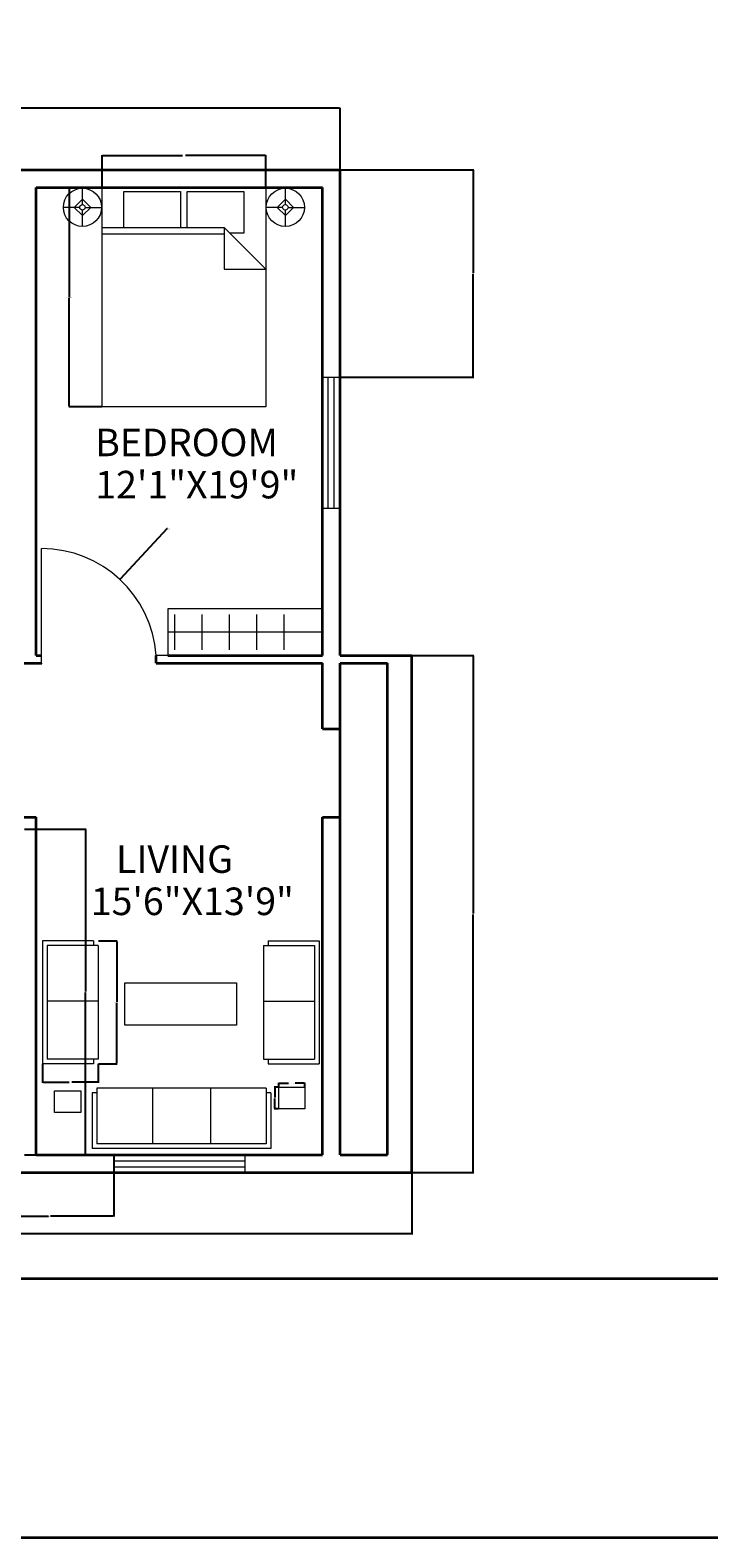
# Model space of a CAD drawing. Units: inches. Extents: x 2286 to 3750, y 1240 to 2345.
# Tile 3 of 7: x 2701 to 2949, y 1240 to 1793. Entities that reach past the tile are written whole.
import ezdxf

# ---------------------------------------------------------------- set-up
doc = ezdxf.new("R2010")
doc.units = ezdxf.units.IN
for name, color, linetype, lineweight in [('A-ANNO-DIMS', 2, 'Continuous', 18), ('A-AREA-IDEN', 7, 'Continuous', 18), ('A-DOOR', 4, 'Continuous', 18), ('A-FLOR-CASE', 8, 'Continuous', 18), ('A-FURN', 8, 'Continuous', 18), ('A-GLAZ', 51, 'Continuous', 18), ('A-WALL', 7, 'Continuous', 35)]:
    doc.layers.add(name, color=color, linetype=linetype, lineweight=lineweight)
doc.styles.get("Standard").update_dxf_attribs({"font": 'arial.ttf'})
doc.dimstyles.get("Standard").update_dxf_attribs({"dimtxt": 0.18, "dimasz": 0.18, "dimexe": 0.18, "dimexo": 0.0625, "dimgap": 0.09, "dimtad": 0, "dimtih": 1, "dimtoh": 1, "dimdec": 4, "dimzin": 0, "dimdsep": 46, "dimtxsty": 'Standard', "dimcen": 0.09, "dimadec": 0, "dimazin": 0, "dimtfac": 1, "dimtdec": 4, "dimtofl": 0, "dimtmove": 0, "dimatfit": 3, "dimfxl": 1, "dimtolj": 1, "dimtzin": 0, "dimarcsym": 0})

# ---------------------------------------------------------------- blocks, each defined once
blk = doc.blocks.new('Bed - Queen')
for p, q in [((0, -80.00003), (0, 0)), ((0, 0), (59.99999, 0)), ((59.99999, 0), (59.99999, -80.00003)), ((7.99999, -1.2), (28.79998, -1.2)), ((7.99999, -14.4), (7.99999, -1.2)), ((28.79998, -1.2), (28.79998, -14.4)), ((31.19999, -1.2), (51.99999, -1.2)), ((31.19999, -14.4), (31.19999, -1.2)), ((51.99999, -1.2), (51.99999, -16.4)), ((0, -14.4), (44.8, -14.4)), ((59.99999, -29.6), (44.8, -14.4)), ((44.8, -14.4), (44.8, -29.6)), ((51.99999, -16.4), (46.79936, -16.4)), ((44.8, -16.8), (0, -16.8)), ((44.8, -29.6), (59.99999, -29.6)), ((59.99999, -80.00003), (0, -80.00003))]:
    blk.add_line(p, q)
blk = doc.blocks.new('Lamp - Table')
for p, q in [((0, 7), (0, 1)), ((-1, 0), (-7, 0)), ((0, 3), (-3, 0)), ((-3, 0), (0, -3)), ((3, 0), (0, 3)), ((0, -3), (3, 0)), ((1, 0), (7, 0)), ((0, -1), (0, -7))]:
    blk.add_line(p, q)
for radius in [7, 1]:
    blk.add_circle((0, 0), radius)
blk = doc.blocks.new('WIN-48x6p5')
for p, q in [((0, 6.51), (0, 0)), ((48, 6.51), (48, 0)), ((0, 4.35), (48, 4.35)), ((0, 2.16), (48, 2.16))]:
    blk.add_line(p, q)
blk = doc.blocks.new('TABLE-END-SMALL')
blk.add_lwpolyline([(9.61, 0), (0, 0), (0, 7.99), (9.61, 7.99)], close=True)
blk = doc.blocks.new('LOVESEAT-2')
for p, q in [((0, 45.01), (0, 0)), ((18.67, 45.01), (0, 45.01)), ((18.67, 45.01), (18.67, 43.31)), ((1.7, 43.31), (1.7, 1.7)), ((20.37, 43.31), (1.7, 43.31)), ((20.37, 43.31), (20.37, 1.7)), ((20.37, 22.95), (1.7, 22.95)), ((18.67, 0), (0, 0)), ((20.37, 1.7), (1.7, 1.7)), ((18.67, 1.7), (18.67, 0))]:
    blk.add_line(p, q)
blk = doc.blocks.new('*D28')
at = {"layer": 'A-ANNO-DIMS', "color": 0, "lineweight": -2, "transparency": 16777216}
for p, q in [((2727.07, 1734.71), (2714.96, 1734.71)), ((2715.14, 1734.53), (2715.14, 1694.9)), ((2715.14, 1654.89), (2715.14, 1694.52)), ((2727.07, 1654.71), (2714.96, 1654.71))]:
    blk.add_line(p, q, dxfattribs=at)
at = {"layer": 'A-ANNO-DIMS', "color": 0, "transparency": 16777216}
for points in [[(2715.11, 1734.53), (2715.17, 1734.53), (2715.14, 1734.71)], [(2715.11, 1654.89), (2715.17, 1654.89), (2715.14, 1654.71)]]:
    blk.add_solid(points, dxfattribs=at)
at = {"layer": 'Defpoints', "color": 0, "transparency": 16777216}
for p in [(2715.14, 1734.71), (2727.14, 1734.71), (2727.14, 1654.71)]:
    blk.add_point(p, dxfattribs=at)
at = {"layer": 'A-ANNO-DIMS', "color": 0, "transparency": 16777216, "insert": (2715.14, 1694.71), "char_height": 0.18, "attachment_point": 5}
blk.add_mtext('\\A1;QUEEN BED 80 TYP.', dxfattribs=at)
blk = doc.blocks.new('*D29')
at = {"layer": 'A-ANNO-DIMS', "color": 0, "lineweight": -2, "transparency": 16777216}
for p, q in [((2727.14, 1734.77), (2727.14, 1746.89)), ((2727.32, 1746.71), (2756.61, 1746.71)), ((2786.96, 1746.71), (2757.67, 1746.71)), ((2787.14, 1734.77), (2787.14, 1746.89))]:
    blk.add_line(p, q, dxfattribs=at)
at = {"layer": 'A-ANNO-DIMS', "color": 0, "transparency": 16777216}
for points in [[(2727.32, 1746.74), (2727.32, 1746.68), (2727.14, 1746.71)], [(2786.96, 1746.74), (2786.96, 1746.68), (2787.14, 1746.71)]]:
    blk.add_solid(points, dxfattribs=at)
at = {"layer": 'Defpoints', "color": 0, "transparency": 16777216}
for p in [(2787.14, 1746.71), (2727.14, 1734.71), (2787.14, 1734.71)]:
    blk.add_point(p, dxfattribs=at)
at = {"layer": 'A-ANNO-DIMS', "color": 0, "transparency": 16777216, "insert": (2757.14, 1746.71), "char_height": 0.18, "attachment_point": 5}
blk.add_mtext('\\A1;60 TYP.', dxfattribs=at)
blk = doc.blocks.new('*D46')
at = {"layer": 'A-ANNO-DIMS', "color": 0, "lineweight": -2, "transparency": 16777216}
for p, q in [((2791.86, 1405.54), (2791.86, 1407.1)), ((2792.04, 1406.92), (2795.41, 1406.92)), ((2801.29, 1406.92), (2797.92, 1406.92)), ((2801.47, 1405.54), (2801.47, 1407.1))]:
    blk.add_line(p, q, dxfattribs=at)
at = {"layer": 'A-ANNO-DIMS', "color": 0, "transparency": 16777216}
for points in [[(2792.04, 1406.95), (2792.04, 1406.89), (2791.86, 1406.92)], [(2801.29, 1406.95), (2801.29, 1406.89), (2801.47, 1406.92)]]:
    blk.add_solid(points, dxfattribs=at)
at = {"layer": 'Defpoints', "color": 0, "transparency": 16777216}
for p in [(2791.86, 1405.48), (2801.47, 1406.92), (2801.47, 1405.48)]:
    blk.add_point(p, dxfattribs=at)
at = {"layer": 'A-ANNO-DIMS', "color": 0, "transparency": 16777216, "insert": (2796.66, 1406.92), "char_height": 0.18, "attachment_point": 5}
blk.add_mtext('\\A1;END TABLE 10 TYP.', dxfattribs=at)
blk = doc.blocks.new('*D47')
at = {"layer": 'A-ANNO-DIMS', "color": 0, "lineweight": -2, "transparency": 16777216}
for p, q in [((2791.79, 1405.48), (2790.24, 1405.48)), ((2790.42, 1405.3), (2790.42, 1401.67)), ((2791.79, 1397.49), (2790.24, 1397.49)), ((2790.42, 1397.67), (2790.42, 1401.3))]:
    blk.add_line(p, q, dxfattribs=at)
at = {"layer": 'A-ANNO-DIMS', "color": 0, "transparency": 16777216}
for points in [[(2790.39, 1405.3), (2790.45, 1405.3), (2790.42, 1405.48)], [(2790.39, 1397.67), (2790.45, 1397.67), (2790.42, 1397.49)]]:
    blk.add_solid(points, dxfattribs=at)
at = {"layer": 'Defpoints', "color": 0, "transparency": 16777216}
for p in [(2790.42, 1405.48), (2791.86, 1405.48), (2791.86, 1397.49)]:
    blk.add_point(p, dxfattribs=at)
at = {"layer": 'A-ANNO-DIMS', "color": 0, "transparency": 16777216, "insert": (2790.42, 1401.48), "char_height": 0.18, "attachment_point": 5}
blk.add_mtext('\\A1;8 TYP.', dxfattribs=at)
blk = doc.blocks.new('*D48')
at = {"layer": 'A-ANNO-DIMS', "color": 0, "lineweight": -2, "transparency": 16777216}
for p, q in [((2725.84, 1459.06), (2732.71, 1459.06)), ((2732.53, 1458.88), (2732.53, 1436.74)), ((2732.53, 1414.23), (2732.53, 1436.37)), ((2725.84, 1414.05), (2732.71, 1414.05))]:
    blk.add_line(p, q, dxfattribs=at)
at = {"layer": 'A-ANNO-DIMS', "color": 0, "transparency": 16777216}
for points in [[(2732.5, 1458.88), (2732.56, 1458.88), (2732.53, 1459.06)], [(2732.5, 1414.23), (2732.56, 1414.23), (2732.53, 1414.05)]]:
    blk.add_solid(points, dxfattribs=at)
at = {"layer": 'Defpoints', "color": 0, "transparency": 16777216}
for p in [(2725.78, 1459.06), (2732.53, 1459.06), (2725.78, 1414.05)]:
    blk.add_point(p, dxfattribs=at)
at = {"layer": 'A-ANNO-DIMS', "color": 0, "transparency": 16777216, "insert": (2732.53, 1436.56), "char_height": 0.18, "attachment_point": 5}
blk.add_mtext('\\A1;LOVESEAT 45 TYP.', dxfattribs=at)
blk = doc.blocks.new('*D49')
at = {"layer": 'A-ANNO-DIMS', "color": 0, "lineweight": -2, "transparency": 16777216}
for p, q in [((2705.4, 1413.99), (2705.4, 1407.12)), ((2725.78, 1413.99), (2725.78, 1407.12)), ((2705.58, 1407.3), (2715.06, 1407.3)), ((2725.6, 1407.3), (2716.12, 1407.3))]:
    blk.add_line(p, q, dxfattribs=at)
at = {"layer": 'A-ANNO-DIMS', "color": 0, "transparency": 16777216}
for points in [[(2705.58, 1407.33), (2705.58, 1407.27), (2705.4, 1407.3)], [(2725.6, 1407.33), (2725.6, 1407.27), (2725.78, 1407.3)]]:
    blk.add_solid(points, dxfattribs=at)
at = {"layer": 'Defpoints', "color": 0, "transparency": 16777216}
for p in [(2705.4, 1414.05), (2725.78, 1414.05), (2725.78, 1407.3)]:
    blk.add_point(p, dxfattribs=at)
at = {"layer": 'A-ANNO-DIMS', "color": 0, "transparency": 16777216, "insert": (2715.59, 1407.3), "char_height": 0.18, "attachment_point": 5}
blk.add_mtext('\\A1;20 TYP.', dxfattribs=at)
blk = doc.blocks.new('*D74')
at = {"layer": 'A-ANNO-DIMS', "color": 0, "lineweight": -2, "transparency": 16777216}
for p, q in [((2405.79, 1374.12), (2405.79, 1351.55)), ((2840.66, 1374.12), (2840.66, 1351.55)), ((2405.97, 1351.73), (2622.83, 1351.73)), ((2840.48, 1351.73), (2623.62, 1351.73))]:
    blk.add_line(p, q, dxfattribs=at)
at = {"layer": 'A-ANNO-DIMS', "color": 0, "transparency": 16777216}
for points in [[(2405.97, 1351.76), (2405.97, 1351.7), (2405.79, 1351.73)], [(2840.48, 1351.76), (2840.48, 1351.7), (2840.66, 1351.73)]]:
    blk.add_solid(points, dxfattribs=at)
at = {"layer": 'Defpoints', "color": 0, "transparency": 16777216}
for p in [(2405.79, 1374.18), (2840.66, 1374.18), (2840.66, 1351.73)]:
    blk.add_point(p, dxfattribs=at)
at = {"layer": 'A-ANNO-DIMS', "color": 0, "transparency": 16777216, "insert": (2623.23, 1351.73), "char_height": 0.18, "attachment_point": 5}
blk.add_mtext('\\A1;434.9', dxfattribs=at)
blk = doc.blocks.new('*D76')
at = {"layer": 'A-ANNO-DIMS', "color": 0, "lineweight": -2, "transparency": 16777216}
for p, q in [((2405.79, 1741.59), (2405.79, 1764.22)), ((2405.97, 1764.04), (2609.67, 1764.04)), ((2814.17, 1764.04), (2610.47, 1764.04)), ((2814.35, 1741.59), (2814.35, 1764.22))]:
    blk.add_line(p, q, dxfattribs=at)
at = {"layer": 'A-ANNO-DIMS', "color": 0, "transparency": 16777216}
for points in [[(2405.97, 1764.07), (2405.97, 1764.01), (2405.79, 1764.04)], [(2814.17, 1764.07), (2814.17, 1764.01), (2814.35, 1764.04)]]:
    blk.add_solid(points, dxfattribs=at)
at = {"layer": 'Defpoints', "color": 0, "transparency": 16777216}
for p in [(2814.35, 1764.04), (2405.79, 1741.53), (2814.35, 1741.53)]:
    blk.add_point(p, dxfattribs=at)
at = {"layer": 'A-ANNO-DIMS', "color": 0, "transparency": 16777216, "insert": (2610.07, 1764.04), "char_height": 0.18, "attachment_point": 5}
blk.add_mtext('\\A1;408.6', dxfattribs=at)
blk = doc.blocks.new('*D77')
at = {"layer": 'A-ANNO-DIMS', "color": 0, "lineweight": -2, "transparency": 16777216}
for p, q in [((2840.73, 1563.64), (2863.29, 1563.64)), ((2863.11, 1563.46), (2863.11, 1469.09)), ((2863.11, 1374.36), (2863.11, 1468.73)), ((2840.73, 1374.18), (2863.29, 1374.18))]:
    blk.add_line(p, q, dxfattribs=at)
at = {"layer": 'A-ANNO-DIMS', "color": 0, "transparency": 16777216}
for points in [[(2863.08, 1563.46), (2863.14, 1563.46), (2863.11, 1563.64)], [(2863.08, 1374.36), (2863.14, 1374.36), (2863.11, 1374.18)]]:
    blk.add_solid(points, dxfattribs=at)
at = {"layer": 'Defpoints', "color": 0, "transparency": 16777216}
for p in [(2840.66, 1563.64), (2863.11, 1563.64), (2840.66, 1374.18)]:
    blk.add_point(p, dxfattribs=at)
at = {"layer": 'A-ANNO-DIMS', "color": 0, "transparency": 16777216, "insert": (2863.11, 1468.91), "char_height": 0.18, "attachment_point": 5}
blk.add_mtext('\\A1;189.46', dxfattribs=at)
blk = doc.blocks.new('*D81')
at = {"layer": 'A-ANNO-DIMS', "color": 0, "lineweight": -2, "transparency": 16777216}
for p, q in [((2698.72, 1500), (2721.28, 1500)), ((2721.1, 1499.82), (2721.1, 1440.53)), ((2721.1, 1380.87), (2721.1, 1440.16)), ((2698.72, 1380.69), (2721.28, 1380.69))]:
    blk.add_line(p, q, dxfattribs=at)
at = {"layer": 'A-ANNO-DIMS', "color": 0, "transparency": 16777216}
for points in [[(2721.07, 1499.82), (2721.13, 1499.82), (2721.1, 1500)], [(2721.07, 1380.87), (2721.13, 1380.87), (2721.1, 1380.69)]]:
    blk.add_solid(points, dxfattribs=at)
at = {"layer": 'Defpoints', "color": 0, "transparency": 16777216}
for p in [(2698.65, 1500), (2698.65, 1380.69), (2721.1, 1380.69)]:
    blk.add_point(p, dxfattribs=at)
at = {"layer": 'A-ANNO-DIMS', "color": 0, "transparency": 16777216, "insert": (2721.1, 1440.35), "char_height": 0.18, "attachment_point": 5}
blk.add_mtext('\\A1;119.32', dxfattribs=at)
blk = doc.blocks.new('*D90')
at = {"layer": 'A-ANNO-DIMS', "color": 0, "lineweight": -2, "transparency": 16777216}
for p, q in [((2684.35, 1380.63), (2684.35, 1358.06)), ((2731.42, 1380.63), (2731.42, 1358.06)), ((2684.53, 1358.24), (2707.49, 1358.24)), ((2731.24, 1358.24), (2708.28, 1358.24))]:
    blk.add_line(p, q, dxfattribs=at)
at = {"layer": 'A-ANNO-DIMS', "color": 0, "transparency": 16777216}
for points in [[(2684.53, 1358.27), (2684.53, 1358.21), (2684.35, 1358.24)], [(2731.24, 1358.27), (2731.24, 1358.21), (2731.42, 1358.24)]]:
    blk.add_solid(points, dxfattribs=at)
at = {"layer": 'Defpoints', "color": 0, "transparency": 16777216}
for p in [(2684.35, 1380.69), (2731.42, 1380.69), (2684.35, 1358.24)]:
    blk.add_point(p, dxfattribs=at)
at = {"layer": 'A-ANNO-DIMS', "color": 0, "transparency": 16777216, "insert": (2707.88, 1358.24), "char_height": 0.18, "attachment_point": 5}
blk.add_mtext('\\A1;47.07', dxfattribs=at)
blk = doc.blocks.new('*D92')
at = {"layer": 'A-ANNO-DIMS', "color": 0, "lineweight": -2, "transparency": 16777216}
for p, q in [((2814.42, 1741.53), (2863.29, 1741.53)), ((2863.11, 1741.35), (2863.11, 1703.7)), ((2863.11, 1665.7), (2863.11, 1703.34)), ((2814.42, 1665.52), (2863.29, 1665.52))]:
    blk.add_line(p, q, dxfattribs=at)
at = {"layer": 'A-ANNO-DIMS', "color": 0, "transparency": 16777216}
for points in [[(2863.08, 1741.35), (2863.14, 1741.35), (2863.11, 1741.53)], [(2863.08, 1665.7), (2863.14, 1665.7), (2863.11, 1665.52)]]:
    blk.add_solid(points, dxfattribs=at)
at = {"layer": 'Defpoints', "color": 0, "transparency": 16777216}
for p in [(2814.35, 1741.53), (2863.11, 1741.53), (2814.35, 1665.52)]:
    blk.add_point(p, dxfattribs=at)
at = {"layer": 'A-ANNO-DIMS', "color": 0, "transparency": 16777216, "insert": (2863.11, 1703.52), "char_height": 0.18, "attachment_point": 5}
blk.add_mtext('\\A1;76.01', dxfattribs=at)
blk = doc.blocks.new('*D129')
at = {"layer": 'A-ANNO-DIMS', "color": 0, "lineweight": -2, "transparency": 16777216}
for p, q in [((2750.9, 1609.95), (2733.81, 1591.59)), ((2751.08, 1609.95), (2750.9, 1609.95)), ((2704.9, 1560.64), (2705.08, 1560.64)), ((2704.99, 1560.55), (2704.99, 1560.73))]:
    blk.add_line(p, q, dxfattribs=at)
at = {"layer": 'A-ANNO-DIMS', "color": 0, "transparency": 16777216}
blk.add_solid([(2733.79, 1591.61), (2733.83, 1591.57), (2733.69, 1591.46)], dxfattribs=at)
at = {"layer": 'Defpoints', "color": 0, "transparency": 16777216}
for p in [(2733.69, 1591.46), (2704.99, 1560.64)]:
    blk.add_point(p, dxfattribs=at)
at = {"layer": 'A-ANNO-DIMS', "color": 0, "transparency": 16777216, "insert": (2751.55, 1609.95), "char_height": 0.18, "attachment_point": 5}
blk.add_mtext('\\A1;R42.11', dxfattribs=at)

msp = doc.modelspace()

# ---------------------------------------------------------------- linework, layer by layer
at = {"layer": 'A-DOOR'}
msp.add_line((2704.9921, 1560.746), (2704.9921, 1602.746), dxfattribs=at)
msp.add_arc((2704.9921, 1560.639), 42.107, 4.084881, 90, dxfattribs=at)
at = {"layer": 'A-FLOR-CASE'}
for p, q in [((2807.8448, 1580.6385), (2751.2518, 1580.6385)), ((2751.2518, 1580.6385), (2751.2518, 1563.6385)), ((2807.8448, 1563.6385), (2807.8448, 1580.6385)), ((2753.8448, 1565.6385), (2753.8448, 1578.6385)), ((2763.8448, 1565.6385), (2763.8448, 1578.6385)), ((2773.8448, 1565.6385), (2773.8448, 1578.6385)), ((2783.8448, 1565.6385), (2783.8448, 1578.6385)), ((2793.8448, 1565.6385), (2793.8448, 1578.6385)), ((2807.8448, 1572.1385), (2751.2518, 1572.1385)), ((2807.8448, 1563.6385), (2746.9921, 1563.6385))]:
    msp.add_line(p, q, dxfattribs=at)
at = {"layer": 'A-FURN'}
for p, q in [((2725.7753, 1457.3613), (2725.7753, 1415.7506)), ((2725.2769, 1403.4385), (2723.5792, 1403.4385)), ((2723.5792, 1403.4385), (2723.5792, 1383.066)), ((2787.2431, 1405.1362), (2725.2769, 1405.1362)), ((2725.2769, 1405.1362), (2725.2769, 1384.7637)), ((2745.6323, 1405.1362), (2745.6323, 1384.7637)), ((2766.8876, 1405.1362), (2766.8876, 1384.7637)), ((2787.2431, 1405.1362), (2787.2431, 1384.7637)), ((2788.9408, 1403.4385), (2787.2431, 1403.4385)), ((2788.9408, 1403.4385), (2788.9408, 1383.066)), ((2788.9408, 1383.066), (2723.5792, 1383.066)), ((2787.2431, 1384.7637), (2725.2769, 1384.7637))]:
    msp.add_line(p, q, dxfattribs=at)
msp.add_lwpolyline([(2776.3518, 1428.2237), (2735.4836, 1428.2237), (2735.4836, 1443.644), (2776.3518, 1443.644)], close=True, dxfattribs=at)
at = {"layer": 'A-WALL'}
for p, q in [((2405.7888, 1741.5266), (2814.3529, 1741.5266)), ((2814.3529, 1563.6385), (2814.3529, 1741.5266)), ((2702.9921, 1563.6385), (2702.9921, 1735.0185)), ((2702.9921, 1735.0185), (2807.8448, 1735.0185)), ((2807.8448, 1563.6385), (2807.8448, 1735.0185)), ((2702.9921, 1563.6385), (2704.9921, 1563.6385)), ((2746.9921, 1560.746), (2746.9921, 1563.6385)), ((2751.2518, 1563.6385), (2807.8448, 1563.6385)), ((2814.3529, 1563.6385), (2840.6637, 1563.6385)), ((2840.6637, 1374.1804), (2840.6637, 1563.6385)), ((2698.6534, 1560.746), (2704.9921, 1560.746)), ((2746.9921, 1560.746), (2807.8448, 1560.746)), ((2807.8448, 1536.746), (2807.8448, 1560.746)), ((2814.3529, 1380.6885), (2814.3529, 1560.746)), ((2814.3529, 1560.746), (2831.6637, 1560.746)), ((2831.6637, 1380.6885), (2831.6637, 1560.746)), ((2807.8448, 1536.746), (2814.3529, 1536.746)), ((2698.6534, 1504.3424), (2702.9921, 1504.3424)), ((2702.9921, 1380.6885), (2702.9921, 1504.3424)), ((2807.8448, 1380.6885), (2807.8448, 1504.3424)), ((2807.8448, 1504.3424), (2814.3529, 1504.3424)), ((2702.9921, 1380.6885), (2807.8448, 1380.6885)), ((2814.3529, 1380.6885), (2831.6637, 1380.6885)), ((2405.7888, 1374.1804), (2840.6637, 1374.1804))]:
    msp.add_line(p, q, dxfattribs=at)
for points in [[(2286.2079, 2344.8717), (3750.2574, 2344.8717), (3750.2574, 1240.4105), (2286.2079, 1240.4105)], [(2354.794, 2286.8809), (3673.7575, 2286.8809), (3673.7575, 1335.3046), (2354.794, 1335.3046)]]:
    msp.add_lwpolyline(points, close=True, dxfattribs=at)

# ---------------------------------------------------------------- block references
at = {"layer": 'A-FURN', "rotation": 180}
for p in [(2719.9852, 1727.742), (2794.3009, 1727.742)]:
    msp.add_blockref('Lamp - Table', p, dxfattribs=at)
at = {"layer": 'A-FURN'}
for name, p in [('Bed - Queen', (2727.1364, 1734.7097)), ('LOVESEAT-2', (2705.4029, 1414.0529)), ('TABLE-END-SMALL', (2709.7859, 1396.2064)), ('TABLE-END-SMALL', (2791.8571, 1397.4897))]:
    msp.add_blockref(name, p, dxfattribs=at)
at = {"layer": 'A-FURN', "extrusion": (0, 0, -1), "zscale": -1}
msp.add_blockref('LOVESEAT-2', (-2806.7062, 1414.0529), dxfattribs=at)
at = {"layer": 'A-GLAZ', "rotation": 89.99999999999841}
msp.add_blockref('WIN-48x6p5', (2814.3529, 1617.5185), dxfattribs=at)
at = {"layer": 'A-GLAZ'}
msp.add_blockref('WIN-48x6p5', (2731.4185, 1374.1804), dxfattribs=at)

# ---------------------------------------------------------------- texts
at = {"layer": 'A-AREA-IDEN'}
for s, height, p in [('BEDROOM', 10.08366, (2724.6503, 1636.5929)), ('12\'1"X19\'9"', 10.083661, (2724.6503, 1621.1386)), ('   LIVING', 10.08366, (2723.0239, 1483.9671)), ('15\'6"X13\'9"', 10.083661, (2723.0239, 1468.5128))]:
    msp.add_text(s, height=height, dxfattribs=at).set_placement(p)

# ---------------------------------------------------------------- dimensions: what is measured, and where the dimension line sits
at = {"layer": 'A-ANNO-DIMS'}
for base, p1, p2, picture, middle in [((2814.3529, 1764.0414), (2405.7888, 1741.5266), (2814.3529, 1741.5266), '*D76', (2610.0709, 1764.0414)), ((2840.6637, 1351.7304), (2405.7888, 1374.1804), (2840.6637, 1374.1804), '*D74', (2623.2262, 1351.7304))]:
    dim = msp.add_linear_dim(base=base, p1=p1, p2=p2, dimstyle='Standard', override={"dimdec": 1, "dimlfac": 1, "dimrnd": 0, "dimzin": 0, "dimdsep": 46, "dimlunit": 2}, dxfattribs=at)
    dim.commit()
    dim.dimension.update_dxf_attribs({"geometry": picture, "text_midpoint": middle})
for base, p1, p2, text, picture, middle in [((2787.1364, 1746.7097), (2727.1364, 1734.7097), (2787.1364, 1734.7097), '<> TYP.', '*D29', (2757.1364, 1746.7097)), ((2725.7753, 1407.3019), (2705.4029, 1414.0529), (2725.7753, 1414.0529), '<> TYP.', '*D49', (2715.5891, 1407.3019)), ((2801.4686, 1406.9202), (2791.8571, 1405.4784), (2801.4686, 1405.4784), 'END TABLE <> TYP.', '*D46', (2796.6629, 1406.9202))]:
    dim = msp.add_linear_dim(base=base, p1=p1, p2=p2, text=text, dimstyle='Standard', override={"dimdec": 0, "dimlfac": 1, "dimrnd": 0, "dimzin": 0, "dimdsep": 46, "dimlunit": 2}, dxfattribs=at)
    dim.commit()
    dim.dimension.update_dxf_attribs({"geometry": picture, "text_midpoint": middle})
for base, p1, p2, angle, picture, middle in [((2863.1137, 1741.5266), (2814.3529, 1665.5185), (2814.3529, 1741.5266), 90, '*D92', (2863.1137, 1703.5225)), ((2863.1137, 1563.6385), (2840.6637, 1374.1804), (2840.6637, 1563.6385), 90, '*D77', (2863.1137, 1468.9094)), ((2721.1034, 1380.6885), (2698.6534, 1500.0037), (2698.6534, 1380.6885), 270, '*D81', (2721.1034, 1440.3461)), ((2684.3514, 1358.2385), (2731.4185, 1380.6885), (2684.3514, 1380.6885), 180, '*D90', (2707.8849, 1358.2385))]:
    dim = msp.add_linear_dim(base=base, p1=p1, p2=p2, angle=angle, dimstyle='Standard', override={"dimdec": 2, "dimlfac": 1, "dimrnd": 0, "dimzin": 0, "dimdsep": 46, "dimlunit": 2}, dxfattribs=at)
    dim.commit()
    dim.dimension.update_dxf_attribs({"geometry": picture, "text_midpoint": middle})
for base, p1, p2, text, picture, middle in [((2715.1364, 1734.7097), (2727.1364, 1654.7096), (2727.1364, 1734.7097), 'QUEEN BED <> TYP.', '*D28', (2715.1364, 1694.7096)), ((2732.5263, 1459.059), (2725.7753, 1414.0529), (2725.7753, 1459.059), 'LOVESEAT <> TYP.', '*D48', (2732.5263, 1436.556)), ((2790.4154, 1405.4784), (2791.8571, 1397.4897), (2791.8571, 1405.4784), '<> TYP.', '*D47', (2790.4154, 1401.4841))]:
    dim = msp.add_linear_dim(base=base, p1=p1, p2=p2, angle=90, text=text, dimstyle='Standard', override={"dimdec": 0, "dimlfac": 1, "dimrnd": 0, "dimzin": 0, "dimdsep": 46, "dimlunit": 2}, dxfattribs=at)
    dim.commit()
    dim.dimension.update_dxf_attribs({"geometry": picture, "text_midpoint": middle})
dim = msp.add_radius_dim(center=(2704.9921, 1560.639), mpoint=(2733.6863, 1591.4553), dimstyle='Standard', override={"dimdec": 2, "dimlfac": 1, "dimrnd": 0, "dimzin": 0, "dimdsep": 46, "dimlunit": 2}, dxfattribs=at)
dim.commit()
dim.dimension.update_dxf_attribs({"geometry": '*D129', "text_midpoint": (2751.5452, 1609.945), "dimtype": 164})

doc.saveas('drawing.dxf')
